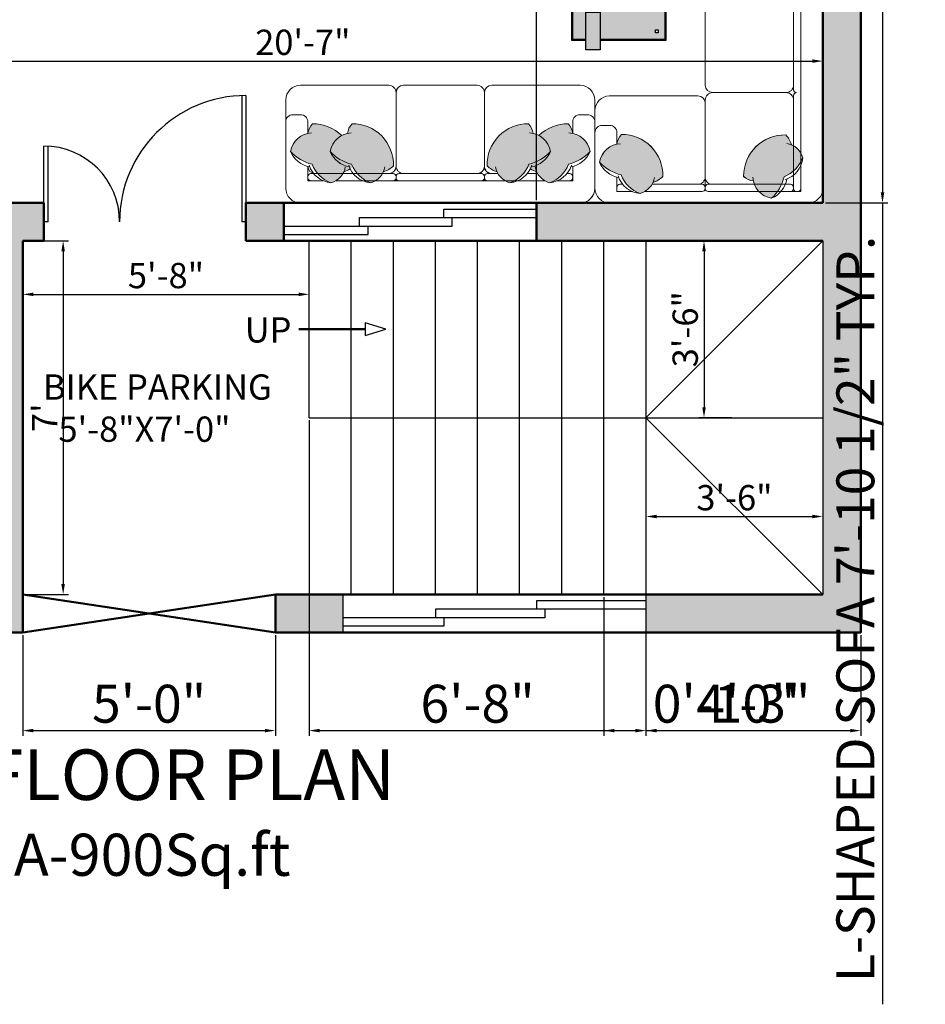
# Model space of a CAD drawing. Units: inches. Extents: x 3274 to 5176, y 1085 to 2172.
# Tile 12 of 16: x 4517 to 4733, y 1085 to 1319. Entities that reach past the tile are written whole.
import ezdxf

# ---------------------------------------------------------------- set-up
doc = ezdxf.new("R2010")
doc.units = ezdxf.units.IN
for name, color, linetype, lineweight in [('A-ANNO-DIMS', 2, 'Continuous', 18), ('A-ANNO-TEXT', 7, 'Continuous', 25), ('A-AREA-IDEN', 3, 'Continuous', 25), ('A-DOOR', 4, 'Continuous', 25), ('A-FLOR-FIXT', 8, 'Continuous', 18), ('A-FLOR-STRS', 7, 'Continuous', 25), ('A-FURN', 8, 'Continuous', 18), ('A-GLAZ', 5, 'Continuous', 25), ('A-WALL', 7, 'Continuous', 50), ('A-WALL-PATT', 8, 'Continuous', 13)]:
    doc.layers.add(name, color=color, linetype=linetype, lineweight=lineweight)
doc.layers.add('MOBIL', color=7, linetype='Continuous')
doc.styles.get("Standard").update_dxf_attribs({"font": 'arial.ttf'})
doc.dimstyles.new('ISO-25', dxfattribs={"dimtxt": 9, "dimasz": 2.5, "dimexe": 1.25, "dimexo": 0.625, "dimtad": 1, "dimdec": 1, "dimlunit": 3, "dimtxsty": 'Standard', "dimcen": 2.5, "dimclrd": 4, "dimclre": 4, "dimclrt": 1, "dimadec": 0, "dimazin": 0, "dimtfac": 1, "dimtdec": 1, "dimtmove": 0, "dimatfit": 3, "dimfxl": 1, "dimarcsym": 0})

# ---------------------------------------------------------------- blocks, each defined once
blk = doc.blocks.new('3')
for p, q in [((47, 30), (47, 0)), ((48, 30), (48, 0)), ((0, 0), (0, 18)), ((1, 0), (1, 18)), ((1, 0), (0, 0)), ((48, 0), (47, 0))]:
    blk.add_line(p, q)
for centre, radius, start, end in [((48, 0), 30, 90, 180), ((0, 0), 18, 0, 90)]:
    blk.add_arc(centre, radius, start, end)
blk = doc.blocks.new('SOFA 1')
at = {"transparency": 33554687}
h = blk.add_hatch(color=256, dxfattribs=at)
h.dxf.hatch_style = 1
h.paths.add_polyline_path([(3769.65, 1307.6, 0.084911), (3767.15, 1309.12, 0.046133), (3766.46, 1311.13), (3759.18, 1311.13, 0.039409), (3758.92, 1310.24, 0.165523), (3756.31, 1309.02, 0.42585), (3767.59, 1297.95, 0.121928), (3769.15, 1300.58, 0.027403), (3769.65, 1300.83)])
h.paths.add_polyline_path([(3765.34, 1313.08), (3760.4, 1313.08, 0.097704), (3759.18, 1311.13), (3766.46, 1311.13, 0.04873)])
h.paths.add_polyline_path([(3763.76, 1314.88, 0.16488), (3760.4, 1313.08), (3765.34, 1313.08, 0.051917)])
h.paths.add_polyline_path([(3771.6, 1305.17, 0.090388), (3769.65, 1307.6), (3769.65, 1300.83, 0.136035), (3771.6, 1302.77)])
h = blk.add_hatch(color=256, dxfattribs=at)
h.dxf.hatch_style = 1
h.paths.add_polyline_path([(3723.52, 1308.63, 0.147724), (3717.76, 1305.24, 0.310469), (3722.42, 1300.4), (3722.42, 1300.25, 0.156703), (3723.62, 1297.8, 0.425821), (3734.69, 1309.08, 0.121928), (3732.05, 1310.63, 0.233216), (3728.6, 1313.59, 0.213835)])
h = blk.add_hatch(color=256, dxfattribs=at)
h.dxf.hatch_style = 1
h.paths.add_polyline_path([(3769.16, 1235.96, 0.122267), (3767.6, 1238.61, 0.425972), (3756.32, 1227.54, 0.165563), (3758.93, 1226.32, 0.309481), (3763.76, 1221.69, 0.002677), (3763.83, 1221.72, 0.146094), (3767.16, 1227.43, 0.212433), (3772.1, 1232.48, 0.235342)])
h = blk.add_hatch(color=256, dxfattribs=at)
h.dxf.hatch_style = 1
h.paths.add_polyline_path([(3769.16, 1225.36, 0.122267), (3767.6, 1228.01, 0.425972), (3756.32, 1216.94, 0.165563), (3758.93, 1215.72, 0.309481), (3763.76, 1211.09, 0.002677), (3763.83, 1211.12, 0.146094), (3767.16, 1216.83, 0.212433), (3772.1, 1221.88, 0.235342)])
for p, q in [((3720.45, 1316.13), (3773.58, 1316.13)), ((3777.51, 1312.19), (3777.51, 1213.72))]:
    blk.add_line(p, q, dxfattribs=at)
for points in [[(3763.76, 1314.88, -0.147724), (3767.15, 1309.12, -0.213355), (3772.1, 1304.05, 0.213355), (3767.15, 1309.12, 0.147724), (3763.76, 1314.88, -0.249545), (3767.86, 1309.77, 0.249545), (3763.77, 1314.89, 0.356779), (3758.8, 1309.23, -0.356779), (3763.76, 1314.88)], [(3717.76, 1305.24, -0.147724), (3723.52, 1308.63, -0.213355), (3728.59, 1313.59, 0.213355), (3723.52, 1308.63, 0.147724), (3717.76, 1305.24, -0.249545), (3722.86, 1309.34, 0.249545), (3717.75, 1305.25, 0.356779), (3723.4, 1300.28, -0.356779), (3717.76, 1305.24)], [(3728.58, 1313.6, -0.306333), (3732.42, 1309.31, 0.306333), (3728.58, 1313.6, 0.306674), (3722.72, 1308.89, -0.306674), (3728.58, 1313.6)], [(3734.69, 1309.08, -0.425972), (3723.62, 1297.8, -0.165552), (3722.4, 1300.4, 0.165552), (3723.62, 1297.79, 0.425972), (3734.69, 1309.07, 0.121514), (3732.07, 1310.63, -0.121514), (3734.69, 1309.08)], [(3767.6, 1297.95, -0.425972), (3756.31, 1309.01, -0.165552), (3758.92, 1310.24, 0.165552), (3756.31, 1309.02, 0.425972), (3767.59, 1297.95, 0.121514), (3769.14, 1300.57, -0.121514), (3767.6, 1297.95)], [(3772.11, 1304.06, -0.306333), (3767.83, 1300.22, 0.306333), (3772.11, 1304.06, 0.306674), (3767.4, 1309.91, -0.306674), (3772.11, 1304.06)], [(3770.44, 1286.63, -0.414214), (3769.66, 1287.4, 0.414214), (3770.44, 1286.63, 0.414214), (3769.66, 1285.83, -0.414214), (3770.44, 1286.63)], [(3748.01, 1262.99, -0.414214), (3746.05, 1264.95, 0.414214), (3748.01, 1262.97, 0.414213), (3746.05, 1261.01, -0.414213), (3748.01, 1262.99)], [(3770.44, 1262.99, -0.414214), (3769.66, 1263.77, 0.414214), (3770.44, 1262.99, 0.414214), (3769.66, 1262.19, -0.414214), (3770.44, 1262.99)], [(3770.83, 1262.97, -0.414214), (3771.61, 1262.19, 0.414214), (3770.83, 1262.99, 0.414214), (3771.61, 1263.77, -0.414214), (3770.83, 1262.97)], [(3748.01, 1239.35, -0.414214), (3746.05, 1241.31, 0.414214), (3748.01, 1239.33, 0.414213), (3746.05, 1237.37, -0.414213), (3748.01, 1239.35)], [(3767.7, 1239.33, -0.414214), (3769.66, 1237.37, 0.414214), (3767.7, 1239.35, 0.414214), (3769.66, 1241.31, -0.414214), (3767.7, 1239.33)], [(3756.32, 1227.54, -0.425972), (3767.6, 1238.61, -0.121514), (3769.16, 1235.98, 0.121514), (3767.6, 1238.61, 0.425972), (3756.32, 1227.54, 0.165552), (3758.93, 1226.32, -0.165552), (3756.32, 1227.54)], [(3770.44, 1239.35, -0.414214), (3769.66, 1240.13, 0.414214), (3770.44, 1239.33, 0.414214), (3769.66, 1238.55, -0.414214), (3770.44, 1239.35)], [(3770.83, 1239.33, -0.414214), (3771.61, 1238.55, 0.414214), (3770.83, 1239.35, 0.414214), (3771.61, 1240.13, -0.414214), (3770.83, 1239.33)], [(3772.1, 1232.5, -0.306674), (3767.41, 1226.64, 0.306674), (3772.1, 1232.5, 0.306333), (3767.84, 1236.34, -0.306333), (3772.1, 1232.5)], [(3763.78, 1221.67, 0.249545), (3767.87, 1226.78, -0.249545), (3763.76, 1221.69, -0.356779), (3758.81, 1227.32, 0.356779), (3763.77, 1221.68, 0.147724), (3767.16, 1227.43, 0.213355), (3772.11, 1232.51, -0.213355), (3767.16, 1227.43, -0.147724), (3763.78, 1221.67)], [(3756.32, 1216.94, -0.200233), (3759.49, 1224.76, 0.200233), (3756.32, 1216.94, 0.165552), (3758.93, 1215.72, -0.165552), (3756.32, 1216.94)], [(3772.1, 1221.9, -0.306674), (3767.41, 1216.04, 0.306674), (3772.1, 1221.9, -0.213355), (3767.16, 1216.83, -0.147724), (3763.77, 1211.08, 0.147724), (3767.15, 1216.83, 0.213355), (3772.1, 1221.9)], [(3763.76, 1211.09, -0.356779), (3758.81, 1216.72, 0.356779), (3763.76, 1211.09, 0.249545), (3767.87, 1216.18, -0.249545), (3763.76, 1211.09)]]:
    blk.add_lwpolyline(points, format="xyb", dxfattribs=at)
for points in [[(3716.51, 1312.2), (3716.51, 1291.44)], [(3722.42, 1313.08), (3722.42, 1309.23), (3722.42, 1313.08), (3726.57, 1313.08)], [(3729.85, 1313.08), (3745.25, 1313.08)], [(3746.01, 1312.3), (3746.01, 1288.55)], [(3768.11, 1313.08), (3746.78, 1313.08)], [(3771.6, 1313.08), (3767.75, 1313.08), (3771.6, 1313.08), (3771.6, 1308.93)], [(3769.66, 1287.39), (3769.65, 1312.3)], [(3771.6, 1313.08), (3771.61, 1233.74)], [(3723.21, 1311.13), (3723.93, 1311.13)], [(3731.82, 1311.13), (3745.25, 1311.13)], [(3746.01, 1310.97), (3746.01, 1311.36)], [(3768.87, 1311.13), (3746.78, 1311.13)], [(3769.65, 1309.43), (3769.65, 1308.71)], [(3746.01, 1288.54), (3746.01, 1308.23)], [(3722.42, 1300.39), (3722.42, 1297.33)], [(3720.45, 1295.38), (3718.48, 1295.38)], [(3720.45, 1287.5), (3744.09, 1287.5)], [(3747.99, 1286.6), (3767.69, 1286.6)], [(3769.66, 1263.75), (3769.66, 1285.81)], [(3746.02, 1284.63), (3746.02, 1264.94)], [(3769.66, 1277.18), (3769.66, 1263.75)], [(3747.99, 1262.97), (3767.69, 1262.97)], [(3769.66, 1240.12), (3769.66, 1262.18)], [(3770.43, 1262.97), (3770.82, 1262.97)], [(3746.02, 1260.99), (3746.02, 1241.3)], [(3747.99, 1239.33), (3767.69, 1239.33)], [(3769.66, 1235.71), (3769.66, 1238.54)], [(3770.43, 1239.33), (3770.82, 1239.33)], [(3746.02, 1237.36), (3746.02, 1213.74)], [(3771.61, 1223.14), (3771.61, 1230.47)], [(3769.66, 1225.11), (3769.66, 1227.82)], [(3767.76, 1215.72), (3771.61, 1215.72), (3771.61, 1219.84), (3771.61, 1215.72)], [(3769.66, 1216.5), (3769.66, 1217.22)], [(3755.86, 1215.72), (3758.92, 1215.72)], [(3753.91, 1211.77), (3753.91, 1213.74)], [(3749.97, 1209.8), (3773.58, 1209.8)]]:
    blk.add_lwpolyline(points, close=True, dxfattribs=at)
for points in [[(3722.42, 1311.91, 0.414214), (3723.2, 1311.13, -0.414214)], [(3770.43, 1313.08, 0.414214), (3769.65, 1312.3, -0.414214)], [(3771.6, 1312.3, 0.414214), (3770.82, 1313.08, -0.414214)], [(3716.51, 1297.34, 0.414214), (3718.47, 1295.38, -0.414214)], [(3720.44, 1295.38, 0.414214), (3722.4, 1297.34, -0.414214)], [(3716.51, 1291.45, 0.414212), (3720.44, 1287.52, -0.414212)], [(3746.03, 1288.56, 0.414214), (3747.99, 1286.6, 0.414213), (3746.03, 1284.64, -0.414213), (3747.99, 1286.6, -0.414214)], [(3769.66, 1284.64, 0.414214), (3767.7, 1286.6, 0.414214), (3769.66, 1288.56, -0.414214), (3767.7, 1286.6, -0.414214)], [(3769.66, 1261.01, 0.414214), (3767.7, 1262.97, 0.414214), (3769.66, 1264.93, -0.414214), (3767.7, 1262.97, -0.414214)], [(3772.13, 1221.9, 0.306333), (3767.84, 1225.74, -0.306333)], [(3769.16, 1225.36, 0.071861), (3768.39, 1227.01, -0.071861)], [(3755.87, 1215.72, 0.414214), (3753.91, 1213.76, -0.414214)], [(3769.66, 1216.52, 0.414214), (3770.44, 1215.74, -0.414214)], [(3770.83, 1215.74, 0.414214), (3771.61, 1216.52, -0.414214)], [(3746.05, 1213.76, 0.414212), (3749.98, 1209.82, -0.414212)], [(3755.87, 1209.8, -0.414214), (3753.91, 1211.76, 0.414214)]]:
    blk.add_lwpolyline(points, format="xyb", close=True, dxfattribs=at)
for centre, radius, start, end in [((3720.44, 1312.2), 3.93, 90.0002, 179.9998), ((3720.44, 1312.19), 3.94, 89.9158, 179.9154), ((3773.58, 1312.2), 3.93, 0.0002, 89.9998), ((3773.57, 1312.19), 3.94, 359.9158, 89.9154), ((3745.22, 1312.29), 0.789, 0.8425, 90.8425), ((3745.24, 1311.91), 0.777, 270, 0), ((3745.24, 1311.91), 0.777, 270, 0), ((3746.8, 1312.29), 0.789, 89.1575, 179.1575), ((3746.79, 1311.91), 0.777, 180, 270), ((3746.79, 1311.91), 0.777, 180, 270), ((3768.87, 1312.3), 0.777, 360, 90), ((3768.87, 1311.91), 0.777, 270, 0), ((3744.09, 1309.21), 1.92, 358.766, 90.5111), ((3747.93, 1309.21), 1.92, 89.4889, 181.234), ((3744.08, 1289.48), 1.96, 270, 360), ((3744.08, 1289.48), 1.96, 270, 360), ((3773.58, 1213.73), 3.93, 270.0002, 359.9998), ((3773.59, 1213.73), 3.93, 269.9156, 359.9152)]:
    blk.add_arc(centre, radius, start, end, dxfattribs=at)
blk = doc.blocks.new('Mesa de centro Cantria feeling')
at = {"layer": 'MOBIL', "ltscale": 0.2}
h = blk.add_hatch(color=256, dxfattribs=at)
h.set_gradient(color1=(74, 55, 38), color2=(104, 77, 54), one_color=1, tint=0.31, name='CYLINDER')
h.paths.add_polyline_path([(-0.85, -0.3), (-0.7, -0.3), (-0.7, 0.1), (-0.85, 0.1)])
h = blk.add_hatch(color=256, dxfattribs=at)
h.set_gradient(color1=(221, 221, 223), one_color=1, tint=1)
h.paths.add_polyline_path([(-0.15, -0.6), (-0.15, -0.89), (-0.01, -0.89), (-0.01, -0.01), (-0.7, -0.01), (-0.7, -0.3), (-0.85, -0.3), (-0.85, -0.01), (-0.99, -0.01), (-0.99, -0.89), (-0.3, -0.89), (-0.3, -0.6)])
h.paths.add_polyline_path([(-0.112, -0.112), (-0.112, -0.082), (-0.082, -0.082), (-0.082, -0.112)], flags=16)
h.paths.add_polyline_path([(-0.888, -0.788), (-0.888, -0.818), (-0.918, -0.818), (-0.918, -0.788)], flags=16)
h = blk.add_hatch(color=256, dxfattribs=at)
h.set_gradient(color1=(74, 55, 38), color2=(104, 77, 54), one_color=1, tint=0.31, name='CYLINDER')
h.paths.add_polyline_path([(-0.15, -0.6), (-0.3, -0.6), (-0.3, -1), (-0.15, -1)])
for points in [[(-0.85, 0), (-1, 0), (-1, -0.9), (-0.3, -0.9)], [(-0.15, -0.9), (0, -0.9), (0, 0), (-0.7, 0)], [(-0.85, -0.01), (-0.99, -0.01), (-0.99, -0.89), (-0.3, -0.89)], [(-0.15, -0.89), (-0.01, -0.89), (-0.01, -0.01), (-0.7, -0.01)]]:
    blk.add_lwpolyline(points, dxfattribs=at)
for points in [[(-0.85, -0.3), (-0.7, -0.3), (-0.7, 0.1), (-0.85, 0.1)], [(-0.082, -0.082), (-0.112, -0.082), (-0.112, -0.112), (-0.082, -0.112)], [(-0.15, -0.6), (-0.3, -0.6), (-0.3, -1), (-0.15, -1)], [(-0.918, -0.818), (-0.888, -0.818), (-0.888, -0.788), (-0.918, -0.788)]]:
    blk.add_lwpolyline(points, close=True, dxfattribs=at)
blk = doc.blocks.new('S1')
at = {"transparency": 33554687}
h = blk.add_hatch(color=256, dxfattribs=at)
h.dxf.hatch_style = 1
h.paths.add_polyline_path([(3706.22, 1117.89, 0.122267), (3708.57, 1119.27, 0.425972), (3698.75, 1129.29, 0.165563), (3697.66, 1126.97, 0.309481), (3693.55, 1122.68, 0.002677), (3693.58, 1122.62, 0.146094), (3698.65, 1119.67, 0.212433), (3703.13, 1115.28, 0.235342)])
h = blk.add_hatch(color=256, dxfattribs=at)
h.dxf.hatch_style = 1
h.paths.add_polyline_path([(3715.63, 1117.89, 0.122267), (3717.98, 1119.27, 0.425972), (3708.16, 1129.29, 0.165563), (3707.07, 1126.97, 0.309481), (3702.96, 1122.68, 0.002677), (3702.99, 1122.62, 0.146094), (3708.06, 1119.67, 0.212433), (3712.54, 1115.28, 0.235342)])
h = blk.add_hatch(color=256, dxfattribs=at)
h.dxf.hatch_style = 1
h.paths.add_polyline_path([(3742.59, 1117.89, -0.122267), (3740.24, 1119.27, -0.425972), (3750.07, 1129.29, -0.165563), (3751.15, 1126.97, -0.309481), (3755.26, 1122.68, -0.002677), (3755.24, 1122.62, -0.146094), (3750.16, 1119.67, -0.212433), (3745.68, 1115.28, -0.235342)])
h = blk.add_hatch(color=256, dxfattribs=at)
h.dxf.hatch_style = 1
h.paths.add_polyline_path([(3752, 1117.89, -0.122267), (3749.65, 1119.27, -0.425972), (3759.48, 1129.29, -0.165563), (3760.56, 1126.97, -0.309481), (3764.67, 1122.68, -0.002677), (3764.65, 1122.62, -0.146094), (3759.57, 1119.67, -0.212433), (3755.09, 1115.28, -0.235342)])
for p, q in [((3747.47, 1115.72), (3704.36, 1115.76)), ((3695.9, 1110.48), (3762.33, 1110.48))]:
    blk.add_line(p, q)
for points in [[(3695.92, 1138.41, 0.414212), (3692.43, 1134.92, -0.414212)], [(3762.3, 1138.41, -0.414212), (3765.79, 1134.92, 0.414212)], [(3692.41, 1129.69, -0.414214), (3694.15, 1131.43, 0.414214)], [(3697.66, 1129.69, 0.414214), (3695.92, 1131.43, -0.414214)], [(3760.56, 1129.69, -0.414214), (3762.3, 1131.43, 0.414214)], [(3765.81, 1129.69, 0.414214), (3764.07, 1131.43, -0.414214)], [(3703.15, 1115.26, 0.306333), (3706.55, 1119.07, -0.306333)], [(3706.22, 1117.89, 0.071861), (3707.68, 1118.58, -0.071861)], [(3720.36, 1117.45, -0.414214), (3718.62, 1119.19, -0.414214), (3716.88, 1117.45, 0.414214), (3718.62, 1119.19, 0.414214)], [(3752, 1117.89, -0.071861), (3750.54, 1118.58, 0.071861)], [(3755.08, 1115.26, -0.306333), (3751.67, 1119.07, 0.306333)], [(3698.37, 1117.45, 0.414214), (3697.68, 1116.76, -0.414214)], [(3697.68, 1116.41, 0.414214), (3698.37, 1115.72, -0.414214)], [(3759.85, 1117.45, -0.414214), (3760.54, 1116.76, 0.414214)], [(3760.54, 1116.41, -0.414214), (3759.85, 1115.72, 0.414214)]]:
    blk.add_lwpolyline(points, format="xyb", close=True, dxfattribs=at)
for points in [[(3695.92, 1138.41), (3716.87, 1138.43)], [(3718.62, 1136.68), (3718.62, 1119.2)], [(3720.37, 1138.43), (3737.85, 1138.43)], [(3739.6, 1136.68), (3739.6, 1119.2)], [(3741.35, 1138.43), (3762.31, 1138.43)], [(3692.41, 1134.93), (3692.41, 1113.97)], [(3692.41, 1134.81), (3692.41, 1113.85)], [(3765.81, 1134.93), (3765.81, 1113.97)], [(3694.16, 1131.43), (3695.91, 1131.43)], [(3697.66, 1129.7), (3697.66, 1126.98)], [(3760.56, 1129.7), (3760.56, 1126.98)], [(3764.06, 1131.43), (3762.31, 1131.43)], [(3697.66, 1119.14), (3697.66, 1115.72), (3701.32, 1115.72), (3697.66, 1115.72)], [(3760.56, 1119.14), (3760.56, 1115.72), (3756.9, 1115.72), (3760.56, 1115.72)], [(3717.92, 1117.45), (3698.34, 1117.45)], [(3698.35, 1117.46), (3698.99, 1117.46)], [(3698.36, 1117.45), (3699, 1117.45)], [(3706, 1117.45), (3717.92, 1117.45)], [(3718.62, 1116.77), (3718.62, 1116.42)], [(3738.9, 1117.45), (3719.32, 1117.45)], [(3739.6, 1116.77), (3739.6, 1116.42)], [(3742.81, 1117.45), (3740.3, 1117.45)], [(3753.97, 1115.72), (3747.47, 1115.72)], [(3752.22, 1117.45), (3749.81, 1117.45)], [(3759.86, 1117.45), (3759.22, 1117.45)]]:
    blk.add_lwpolyline(points, close=True, dxfattribs=at)
for points in [[(3718.6, 1136.67, 0.414214), (3716.86, 1138.41, -0.414214), (3718.62, 1136.67, -0.414213), (3720.36, 1138.41, 0.414213), (3718.6, 1136.67)], [(3739.58, 1136.67, 0.414214), (3737.84, 1138.41, -0.414214), (3739.6, 1136.67, -0.414213), (3741.34, 1138.41, 0.414213), (3739.58, 1136.67)], [(3698.75, 1129.29, -0.200233), (3705.69, 1126.47, 0.200233), (3698.75, 1129.29, 0.165552), (3697.66, 1126.97, -0.165552), (3698.75, 1129.29)], [(3708.16, 1129.29, -0.425972), (3717.98, 1119.27, -0.121514), (3715.65, 1117.89, 0.121514), (3717.98, 1119.27, 0.425972), (3708.16, 1129.29, 0.165552), (3707.07, 1126.97, -0.165552), (3708.16, 1129.29)], [(3750.07, 1129.29, 0.425972), (3740.24, 1119.27, 0.121514), (3742.57, 1117.89, -0.121514), (3740.24, 1119.27, -0.425972), (3750.07, 1129.29, -0.165552), (3751.15, 1126.97, 0.165552), (3750.07, 1129.29)], [(3759.48, 1129.29, 0.200233), (3752.53, 1126.47, -0.200233), (3759.48, 1129.29, -0.165552), (3760.56, 1126.97, 0.165552), (3759.48, 1129.29)], [(3693.55, 1122.68, -0.356779), (3698.55, 1127.08, 0.356779), (3693.55, 1122.68, 0.249545), (3698.07, 1119.04, -0.249545), (3693.55, 1122.68)], [(3702.94, 1122.67, 0.249545), (3707.48, 1119.04, -0.249545), (3702.96, 1122.68, -0.356779), (3707.96, 1127.08, 0.356779), (3702.95, 1122.67, 0.147724), (3708.06, 1119.67, 0.213355), (3712.56, 1115.27, -0.213355), (3708.06, 1119.67, -0.147724), (3702.94, 1122.67)], [(3755.28, 1122.67, -0.249545), (3750.74, 1119.04, 0.249545), (3755.26, 1122.68, 0.356779), (3750.26, 1127.08, -0.356779), (3755.27, 1122.67, -0.147724), (3750.16, 1119.67, -0.213355), (3745.66, 1115.27, 0.213355), (3750.16, 1119.67, 0.147724), (3755.28, 1122.67)], [(3764.67, 1122.68, 0.356779), (3759.67, 1127.08, -0.356779), (3764.67, 1122.68, -0.249545), (3760.15, 1119.04, 0.249545), (3764.67, 1122.68)], [(3703.15, 1115.28, -0.306674), (3697.95, 1119.44, 0.306674), (3703.15, 1115.28, -0.213355), (3698.65, 1119.67, -0.147724), (3693.54, 1122.67, 0.147724), (3698.65, 1119.67, 0.213355), (3703.15, 1115.28)], [(3755.07, 1115.28, 0.306674), (3760.27, 1119.44, -0.306674), (3755.07, 1115.28, 0.213355), (3759.57, 1119.67, 0.147724), (3764.68, 1122.67, -0.147724), (3759.57, 1119.67, -0.213355), (3755.07, 1115.28)], [(3712.56, 1115.28, -0.306674), (3707.36, 1119.44, 0.306674), (3712.56, 1115.28, 0.306333), (3715.96, 1119.07, -0.306333), (3712.56, 1115.28)], [(3739.6, 1119.19, 0.414214), (3741.34, 1117.45, -0.414214), (3739.58, 1119.19, -0.414214), (3737.84, 1117.45, 0.414214), (3739.6, 1119.19)], [(3745.66, 1115.28, 0.306674), (3750.86, 1119.44, -0.306674), (3745.66, 1115.28, -0.306333), (3742.26, 1119.07, 0.306333), (3745.66, 1115.28)], [(3718.6, 1116.76, 0.414214), (3717.91, 1117.45, -0.414214), (3718.6, 1116.76, -0.414214), (3719.31, 1117.45, 0.414214), (3718.6, 1116.76)], [(3718.62, 1116.41, 0.414214), (3719.31, 1115.72, -0.414214), (3718.6, 1116.41, -0.414214), (3717.91, 1115.72, 0.414214), (3718.62, 1116.41)], [(3739.58, 1116.76, 0.414214), (3738.89, 1117.45, -0.414214), (3739.6, 1116.76, -0.414214), (3740.29, 1117.45, 0.414214), (3739.58, 1116.76)], [(3739.6, 1116.41, 0.414214), (3740.29, 1115.72, -0.414214), (3739.58, 1116.41, -0.414214), (3738.89, 1115.72, 0.414214), (3739.6, 1116.41)]]:
    blk.add_lwpolyline(points, format="xyb", dxfattribs=at)
for centre, radius, start, end in [((3699.38, 1119.19), 1.74, 180, 270), ((3699.38, 1119.19), 1.74, 180, 270), ((3695.9, 1113.97), 3.5, 180.0846, 270.0842), ((3762.32, 1113.97), 3.49, 270.0002, 359.9998), ((3762.33, 1113.96), 3.48, 270.0848, 0.0844)]:
    blk.add_arc(centre, radius, start, end, dxfattribs=at)
blk = doc.blocks.new('*D77')
at = {"layer": 'A-ANNO-DIMS', "color": 0, "lineweight": -2, "transparency": 16777216}
for p, q in [((4518.81, 1266.35), (4529.02, 1266.35)), ((4527.77, 1263.85), (4527.77, 1184.85)), ((4518.81, 1182.35), (4529.02, 1182.35))]:
    blk.add_line(p, q, dxfattribs=at)
at = {"layer": 'A-ANNO-DIMS', "color": 0, "transparency": 16777216}
for points in [[(4527.35, 1263.85), (4528.19, 1263.85), (4527.77, 1266.35)], [(4527.35, 1184.85), (4528.19, 1184.85), (4527.77, 1182.35)]]:
    blk.add_solid(points, dxfattribs=at)
at = {"layer": 'Defpoints', "color": 0, "transparency": 16777216}
for p in [(4518.19, 1266.35), (4518.19, 1182.35), (4527.77, 1182.35)]:
    blk.add_point(p, dxfattribs=at)
at = {"layer": 'A-ANNO-DIMS', "color": 0, "transparency": 16777216, "insert": (4524.15, 1224.35), "char_height": 6, "attachment_point": 5, "rotation": 90}
blk.add_mtext("7'", dxfattribs=at)
blk = doc.blocks.new('*D78')
at = {"layer": 'A-ANNO-DIMS', "color": 0, "lineweight": -2, "transparency": 16777216}
for p, q in [((4520.69, 1253.63), (4583.69, 1253.63)), ((4586.19, 1254.26), (4586.19, 1254.88)), ((4518.19, 1253.01), (4518.19, 1252.38))]:
    blk.add_line(p, q, dxfattribs=at)
at = {"layer": 'A-ANNO-DIMS', "color": 0, "transparency": 16777216}
for points in [[(4520.69, 1254.05), (4520.69, 1253.22), (4518.19, 1253.63)], [(4583.69, 1254.05), (4583.69, 1253.22), (4586.19, 1253.63)]]:
    blk.add_solid(points, dxfattribs=at)
at = {"layer": 'Defpoints', "color": 0, "transparency": 16777216}
for p in [(4518.19, 1253.63), (4586.19, 1253.63), (4586.19, 1253.63)]:
    blk.add_point(p, dxfattribs=at)
at = {"layer": 'A-ANNO-DIMS', "color": 0, "transparency": 16777216, "insert": (4552.19, 1257.32), "char_height": 6, "attachment_point": 5}
blk.add_mtext('5\'-8"', dxfattribs=at)
blk = doc.blocks.new('*D79')
at = {"layer": 'A-ANNO-DIMS', "color": 0, "lineweight": -2, "transparency": 16777216}
for p, q in [((4686.6, 1266.35), (4678.72, 1266.35)), ((4679.97, 1263.85), (4679.97, 1226.85)), ((4686.6, 1224.35), (4678.72, 1224.35))]:
    blk.add_line(p, q, dxfattribs=at)
at = {"layer": 'A-ANNO-DIMS', "color": 0, "transparency": 16777216}
for points in [[(4679.56, 1263.85), (4680.39, 1263.85), (4679.97, 1266.35)], [(4679.56, 1226.85), (4680.39, 1226.85), (4679.97, 1224.35)]]:
    blk.add_solid(points, dxfattribs=at)
at = {"layer": 'Defpoints', "color": 0, "transparency": 16777216}
for p in [(4687.22, 1266.35), (4679.97, 1224.35), (4687.22, 1224.35)]:
    blk.add_point(p, dxfattribs=at)
at = {"layer": 'A-ANNO-DIMS', "color": 0, "transparency": 16777216, "insert": (4676.28, 1245.35), "char_height": 6, "attachment_point": 5, "rotation": 90}
blk.add_mtext('3\'-6"', dxfattribs=at)
blk = doc.blocks.new('*D80')
at = {"layer": 'A-ANNO-DIMS', "color": 0, "lineweight": -2, "transparency": 16777216}
for p, q in [((4666.19, 1204.4), (4666.19, 1199.64)), ((4708.19, 1204.4), (4708.19, 1199.64)), ((4668.69, 1200.89), (4705.69, 1200.89))]:
    blk.add_line(p, q, dxfattribs=at)
at = {"layer": 'A-ANNO-DIMS', "color": 0, "transparency": 16777216}
for points in [[(4668.69, 1201.31), (4668.69, 1200.47), (4666.19, 1200.89)], [(4705.69, 1201.31), (4705.69, 1200.47), (4708.19, 1200.89)]]:
    blk.add_solid(points, dxfattribs=at)
at = {"layer": 'Defpoints', "color": 0, "transparency": 16777216}
for p in [(4666.19, 1205.03), (4708.19, 1205.03), (4708.19, 1200.89)]:
    blk.add_point(p, dxfattribs=at)
at = {"layer": 'A-ANNO-DIMS', "color": 0, "transparency": 16777216, "insert": (4687.19, 1204.58), "char_height": 6, "attachment_point": 5}
blk.add_mtext('3\'-6"', dxfattribs=at)
blk = doc.blocks.new('*D81')
at = {"layer": 'A-ANNO-DIMS', "color": 0, "lineweight": -2, "transparency": 16777216}
for p, q in [((4461.19, 1312.95), (4461.19, 1307.77)), ((4708.19, 1312.95), (4708.19, 1307.77)), ((4463.69, 1309.02), (4705.69, 1309.02))]:
    blk.add_line(p, q, dxfattribs=at)
at = {"layer": 'A-ANNO-DIMS', "color": 0, "transparency": 16777216}
for points in [[(4463.69, 1309.44), (4463.69, 1308.61), (4461.19, 1309.02)], [(4705.69, 1309.44), (4705.69, 1308.61), (4708.19, 1309.02)]]:
    blk.add_solid(points, dxfattribs=at)
at = {"layer": 'Defpoints', "color": 0, "transparency": 16777216}
for p in [(4461.19, 1313.57), (4708.19, 1313.57), (4708.19, 1309.02)]:
    blk.add_point(p, dxfattribs=at)
at = {"layer": 'A-ANNO-DIMS', "color": 0, "transparency": 16777216, "insert": (4584.69, 1312.71), "char_height": 6, "attachment_point": 5}
blk.add_mtext('20\'-7"', dxfattribs=at)
blk = doc.blocks.new('WIN-60')
for p, q in [((4598.19, 1271.85), (4640.19, 1271.85)), ((4598.19, 1269.85), (4598.19, 1271.85)), ((4618.19, 1273.85), (4640.19, 1273.85)), ((4618.19, 1271.85), (4618.19, 1273.85)), ((4620.19, 1269.85), (4620.19, 1271.85)), ((4580.19, 1269.85), (4620.19, 1269.85)), ((4600.19, 1267.85), (4600.19, 1269.85)), ((4580.19, 1267.85), (4600.19, 1267.85))]:
    blk.add_line(p, q)
blk = doc.blocks.new('WIN-72')
for p, q in [((4462.19, 1180.85), (4436.19, 1180.85)), ((4436.19, 1180.85), (4436.19, 1178.85)), ((4462.19, 1178.85), (4412.19, 1178.85)), ((4412.19, 1178.85), (4412.19, 1176.85)), ((4438.19, 1178.85), (4438.19, 1176.85)), ((4438.19, 1176.85), (4390.19, 1176.85)), ((4414.19, 1176.85), (4414.19, 1174.85)), ((4414.19, 1174.85), (4390.19, 1174.85))]:
    blk.add_line(p, q)
blk = doc.blocks.new('*D136')
at = {"layer": 'A-ANNO-DIMS', "color": 4, "lineweight": -2, "transparency": 16777216}
for p, q in [((4708.83, 1369.73), (4723.61, 1369.73)), ((4722.36, 1367.23), (4722.36, 1277.84)), ((4708.83, 1275.34), (4723.61, 1275.34)), ((4722.36, 1275.34), (4722.36, 1085.06))]:
    blk.add_line(p, q, dxfattribs=at)
at = {"layer": 'A-ANNO-DIMS', "color": 4, "transparency": 16777216}
for points in [[(4721.94, 1367.23), (4722.78, 1367.23), (4722.36, 1369.73)], [(4721.94, 1277.84), (4722.78, 1277.84), (4722.36, 1275.34)]]:
    blk.add_solid(points, dxfattribs=at)
at = {"layer": 'Defpoints', "color": 0, "transparency": 16777216}
for p in [(4708.2, 1369.73), (4708.2, 1275.34), (4722.36, 1275.34)]:
    blk.add_point(p, dxfattribs=at)
at = {"layer": 'A-ANNO-DIMS', "color": 1, "transparency": 16777216, "insert": (4717.08, 1178.95), "char_height": 9, "attachment_point": 5, "rotation": 90}
blk.add_mtext('L-SHAPED SOFA 7\'-10 1/2" TYP.', dxfattribs=at)
blk = doc.blocks.new('*D148')
at = {"layer": 'A-ANNO-DIMS', "color": 4, "lineweight": -2, "transparency": 16777216}
for p, q in [((4666.19, 1172.73), (4666.19, 1148.8)), ((4717.19, 1172.73), (4717.19, 1148.8)), ((4668.69, 1150.05), (4714.69, 1150.05))]:
    blk.add_line(p, q, dxfattribs=at)
at = {"layer": 'A-ANNO-DIMS', "color": 4, "transparency": 16777216}
for points in [[(4668.69, 1150.47), (4668.69, 1149.64), (4666.19, 1150.05)], [(4714.69, 1150.47), (4714.69, 1149.64), (4717.19, 1150.05)]]:
    blk.add_solid(points, dxfattribs=at)
at = {"layer": 'Defpoints', "color": 0, "transparency": 16777216}
for p in [(4666.19, 1173.35), (4717.19, 1173.35), (4717.19, 1150.05)]:
    blk.add_point(p, dxfattribs=at)
at = {"layer": 'A-ANNO-DIMS', "color": 1, "transparency": 16777216, "insert": (4691.69, 1155.28), "char_height": 9, "attachment_point": 5}
blk.add_mtext('4\'-3"', dxfattribs=at)
blk = doc.blocks.new('*D149')
at = {"layer": 'A-ANNO-DIMS', "color": 4, "lineweight": -2, "transparency": 16777216}
for p, q in [((4518.19, 1172.73), (4518.19, 1148.8)), ((4578.19, 1172.73), (4578.19, 1148.8)), ((4520.69, 1150.05), (4575.69, 1150.05))]:
    blk.add_line(p, q, dxfattribs=at)
at = {"layer": 'A-ANNO-DIMS', "color": 4, "transparency": 16777216}
for points in [[(4520.69, 1150.47), (4520.69, 1149.64), (4518.19, 1150.05)], [(4575.69, 1150.47), (4575.69, 1149.64), (4578.19, 1150.05)]]:
    blk.add_solid(points, dxfattribs=at)
at = {"layer": 'Defpoints', "color": 0, "transparency": 16777216}
for p in [(4518.19, 1173.35), (4578.19, 1173.35), (4578.19, 1150.05)]:
    blk.add_point(p, dxfattribs=at)
at = {"layer": 'A-ANNO-DIMS', "color": 1, "transparency": 16777216, "insert": (4548.19, 1155.27), "char_height": 9, "attachment_point": 5}
blk.add_mtext('5\'-0"', dxfattribs=at)
blk = doc.blocks.new('*D152')
at = {"layer": 'A-ANNO-DIMS', "color": 4, "lineweight": -2, "transparency": 16777216}
for p, q in [((4586.19, 1223.73), (4586.19, 1148.8)), ((4666.19, 1223.73), (4666.19, 1148.8)), ((4588.69, 1150.05), (4663.69, 1150.05))]:
    blk.add_line(p, q, dxfattribs=at)
at = {"layer": 'A-ANNO-DIMS', "color": 4, "transparency": 16777216}
for points in [[(4588.69, 1150.47), (4588.69, 1149.64), (4586.19, 1150.05)], [(4663.69, 1150.47), (4663.69, 1149.64), (4666.19, 1150.05)]]:
    blk.add_solid(points, dxfattribs=at)
at = {"layer": 'Defpoints', "color": 0, "transparency": 16777216}
for p in [(4586.19, 1224.35), (4666.19, 1224.35), (4666.19, 1150.05)]:
    blk.add_point(p, dxfattribs=at)
at = {"layer": 'A-ANNO-DIMS', "color": 1, "transparency": 16777216, "insert": (4626.19, 1155.27), "char_height": 9, "attachment_point": 5}
blk.add_mtext('6\'-8"', dxfattribs=at)
blk = doc.blocks.new('*D153')
at = {"layer": 'A-ANNO-DIMS', "color": 4, "lineweight": -2, "transparency": 16777216}
for p, q in [((4656.19, 1181.73), (4656.19, 1148.8)), ((4666.19, 1181.73), (4666.19, 1148.8)), ((4658.69, 1150.05), (4663.69, 1150.05)), ((4666.19, 1150.05), (4700.85, 1150.05))]:
    blk.add_line(p, q, dxfattribs=at)
at = {"layer": 'A-ANNO-DIMS', "color": 4, "transparency": 16777216}
for points in [[(4658.69, 1150.47), (4658.69, 1149.64), (4656.19, 1150.05)], [(4663.69, 1150.47), (4663.69, 1149.64), (4666.19, 1150.05)]]:
    blk.add_solid(points, dxfattribs=at)
at = {"layer": 'Defpoints', "color": 0, "transparency": 16777216}
for p in [(4656.19, 1182.35), (4666.19, 1182.35), (4666.19, 1150.05)]:
    blk.add_point(p, dxfattribs=at)
at = {"layer": 'A-ANNO-DIMS', "color": 1, "transparency": 16777216, "insert": (4684.77, 1155.27), "char_height": 9, "attachment_point": 5}
blk.add_mtext('0\'-10"', dxfattribs=at)
blk = doc.blocks.new('*D154')
at = {"layer": 'A-ANNO-DIMS', "color": 4, "lineweight": -2, "transparency": 16777216}
for p, q in [((4640.19, 1275.98), (4640.19, 1557.9)), ((4708.19, 1275.98), (4708.19, 1557.9)), ((4642.69, 1556.65), (4705.69, 1556.65))]:
    blk.add_line(p, q, dxfattribs=at)
at = {"layer": 'A-ANNO-DIMS', "color": 4, "transparency": 16777216}
for points in [[(4642.69, 1557.07), (4642.69, 1556.24), (4640.19, 1556.65)], [(4705.69, 1557.07), (4705.69, 1556.24), (4708.19, 1556.65)]]:
    blk.add_solid(points, dxfattribs=at)
at = {"layer": 'Defpoints', "color": 0, "transparency": 16777216}
for p in [(4708.19, 1556.65), (4640.19, 1275.35), (4708.19, 1275.35)]:
    blk.add_point(p, dxfattribs=at)
at = {"layer": 'A-ANNO-DIMS', "color": 1, "transparency": 16777216, "insert": (4674.19, 1561.87), "char_height": 9, "attachment_point": 5}
blk.add_mtext('5\'-8"', dxfattribs=at)

msp = doc.modelspace()

# ---------------------------------------------------------------- hatches: boundary and pattern name
at = {"layer": 'A-WALL-PATT'}
h = msp.add_hatch(color=256, dxfattribs=at)
h.dxf.hatch_style = 1
h.paths.add_polyline_path([(4717.19, 1533.35), (4357.19, 1533.35), (4357.19, 1173.35), (4390.19, 1173.35), (4390.19, 1182.35), (4366.19, 1182.35), (4366.19, 1266.35), (4426.19, 1266.35), (4426.19, 1271.35), (4366.19, 1271.35), (4366.19, 1375.35), (4426.19, 1375.35), (4426.19, 1380.35), (4366.19, 1380.35), (4366.19, 1524.35), (4708.19, 1524.35), (4708.19, 1380.35), (4578.19, 1380.35), (4578.19, 1375.35), (4708.19, 1375.35), (4708.19, 1275.35), (4640.19, 1275.35), (4640.19, 1266.35), (4708.19, 1266.35), (4708.19, 1182.35), (4666.19, 1182.35), (4666.19, 1173.35), (4717.19, 1173.35)])
h.paths.add_polyline_path([(4461.19, 1375.35), (4477.19, 1375.35), (4477.19, 1380.35), (4456.19, 1380.35), (4456.19, 1319.35), (4401.19, 1319.35), (4401.19, 1339.35), (4396.19, 1339.35), (4396.19, 1314.35), (4456.19, 1314.35), (4456.19, 1266.35), (4477.19, 1266.35), (4477.19, 1271.35), (4461.19, 1271.35)], flags=17)
h.paths.add_polyline_path([(4518.19, 1483.35), (4536.19, 1483.35), (4536.19, 1488.35), (4513.19, 1488.35), (4513.19, 1375.35), (4536.19, 1375.35), (4536.19, 1380.35), (4518.19, 1380.35), (4518.19, 1418.35), (4548.19, 1418.35), (4548.19, 1423.35), (4518.19, 1423.35)], flags=17)
h.paths.add_polyline_path([(4583.19, 1488.35), (4560.19, 1488.35), (4560.19, 1483.35), (4578.19, 1483.35), (4578.19, 1416.35), (4583.19, 1416.35)], flags=17)
h.paths.add_polyline_path([(4518.19, 1266.35), (4523.19, 1266.35), (4523.19, 1275.35), (4513.19, 1275.35), (4513.19, 1182.35), (4462.19, 1182.35), (4462.19, 1173.35), (4518.19, 1173.35)], flags=17)
h.paths.add_polyline_path([(4580.19, 1275.35), (4571.19, 1275.35), (4571.19, 1270.85), (4571.19, 1266.35), (4580.19, 1266.35)], flags=17)
h.paths.add_polyline_path([(4594.19, 1182.35), (4578.19, 1182.35), (4578.19, 1173.35), (4594.19, 1173.35)], flags=17)
h.paths.add_polyline_path([(4573.24, 1316.29), (4647.44, 1316.29), (4647.44, 1346.14), (4573.24, 1346.14)], flags=25)
h.paths.add_polyline_path([(4529.43, 1453), (4568.61, 1453), (4568.61, 1475.39), (4529.43, 1475.39)], flags=25)
h.paths.add_polyline_path([(4619, 1443.76), (4687.39, 1443.76), (4687.39, 1473.61), (4619, 1473.61)], flags=25)
h.paths.add_polyline_path([(4527.67, 1497.04), (4569.64, 1497.04), (4569.64, 1519.43), (4527.67, 1519.43)], flags=25)
h.paths.add_polyline_path([(4407.08, 1443.76), (4475.47, 1443.76), (4475.47, 1473.61), (4407.08, 1473.61)], flags=25)

# ---------------------------------------------------------------- linework, layer by layer
at = {"layer": 'A-FLOR-STRS'}
for p, q in [((4586.19, 1224.35), (4586.19, 1266.35)), ((4596.19, 1224.35), (4596.19, 1266.35)), ((4606.19, 1224.35), (4606.19, 1266.35)), ((4616.19, 1224.35), (4616.19, 1266.35)), ((4626.19, 1224.35), (4626.19, 1266.35)), ((4636.19, 1224.35), (4636.19, 1266.35)), ((4646.19, 1224.35), (4646.19, 1266.35)), ((4656.19, 1224.35), (4656.19, 1266.35)), ((4666.19, 1266.35), (4666.19, 1182.35)), ((4666.19, 1224.35), (4708.19, 1266.35)), ((4708.19, 1266.35), (4708.19, 1182.35)), ((4586.19, 1224.35), (4708.19, 1224.35)), ((4596.19, 1182.35), (4596.19, 1224.35)), ((4606.19, 1182.35), (4606.19, 1224.35)), ((4616.19, 1182.35), (4616.19, 1224.35)), ((4626.19, 1182.35), (4626.19, 1224.35)), ((4636.19, 1182.35), (4636.19, 1224.35)), ((4646.19, 1182.35), (4646.19, 1224.35)), ((4656.19, 1182.35), (4656.19, 1224.35)), ((4666.19, 1224.35), (4708.19, 1182.35)), ((4594.19, 1182.35), (4594.19, 1173.35)), ((4666.19, 1182.35), (4666.19, 1173.35))]:
    msp.add_line(p, q, dxfattribs=at)
msp.add_lwpolyline([(4604.39, 1245.35), (4599.5, 1246.85), (4599.5, 1243.86)], close=True, dxfattribs=at)
at = {"layer": 'A-WALL'}
for p, q in [((4708.19, 1375.35), (4708.19, 1275.35)), ((4513.19, 1275.35), (4523.19, 1275.35)), ((4523.19, 1266.35), (4523.19, 1275.35)), ((4571.19, 1266.35), (4571.19, 1275.35)), ((4571.19, 1275.35), (4708.19, 1275.35)), ((4580.19, 1266.35), (4580.19, 1275.35)), ((4640.19, 1266.35), (4640.19, 1275.35)), ((4518.19, 1173.35), (4518.19, 1266.35)), ((4518.19, 1266.35), (4523.19, 1266.35)), ((4571.19, 1266.35), (4708.19, 1266.35)), ((4583.75, 1245.35), (4599.5, 1245.35)), ((4518.19, 1173.35), (4578.19, 1182.35)), ((4578.19, 1173.35), (4518.19, 1182.35)), ((4708.19, 1182.35), (4578.19, 1182.35)), ((4578.19, 1173.35), (4578.19, 1182.35))]:
    msp.add_line(p, q, dxfattribs=at)
msp.add_lwpolyline([(4518.19, 1173.35), (4357.19, 1173.35), (4357.19, 1533.35), (4717.19, 1533.35), (4717.19, 1173.35), (4578.19, 1173.35)], dxfattribs=at)

# ---------------------------------------------------------------- block references
at = {"layer": 'A-DOOR'}
msp.add_blockref('3', (4523.19, 1270.85), dxfattribs=at)
at = {"layer": 'A-FLOR-FIXT'}
msp.add_blockref('S1', (888.23, 164.87), dxfattribs=at)
at = {"layer": 'A-FURN', "rotation": 180}
for name, p, xscale, yscale, zscale in [('SOFA 1', (1355.08, 2443.61), -0.887653230693335, 0.887653230693335, 0.887653230693335), ('Mesa de centro Cantria feeling', (4670.91, 1313.94), -22.3138190187957, 22.3138190187957, 22.3138190187957)]:
    msp.add_blockref(name, p, dxfattribs=dict(at, xscale=xscale, yscale=yscale, zscale=zscale))
at = {"layer": 'A-GLAZ'}
for name, p in [('WIN-60', (0, 0)), ('WIN-72', (204, 0))]:
    msp.add_blockref(name, p, dxfattribs=at)

# ---------------------------------------------------------------- texts
at = {"layer": 'A-ANNO-TEXT'}
msp.add_text('UP', height=6, dxfattribs=at).set_placement((4570.9, 1242.2))
at = {"layer": 'A-ANNO-TEXT', "insert": (4436.88, 1145.58), "char_height": 12, "attachment_point": 1}
msp.add_mtext_dynamic_manual_height_columns('GROUND FLOOR PLAN\\P{\\H0.83333x;      SLAB AREA-900Sq.ft}', width=202.3193, gutter_width=30, heights=[0], dxfattribs=at)
at = {"layer": 'A-AREA-IDEN', "insert": (4522.99, 1234.63), "char_height": 6, "attachment_point": 1}
msp.add_mtext_dynamic_manual_height_columns('BIKE PARKING\\P  5\'-8"X7\'-0"', width=58.0121, gutter_width=30, heights=[0], dxfattribs=at)

# ---------------------------------------------------------------- dimensions: what is measured, and where the dimension line sits
at = {"layer": 'A-ANNO-DIMS'}
for base, p1, p2, override, picture, middle in [((4708.19, 1556.65), (4640.19, 1275.35), (4708.19, 1275.35), {"dimdec": 1, "dimlfac": 1, "dimrnd": 0, "dimzin": 1, "dimdsep": 46, "dimlunit": 4, "dimfrac": 2}, '*D154', (4674.19, 1561.87)), ((4708.19, 1309.02), (4461.19, 1313.57), (4708.19, 1313.57), {"dimtxt": 6, "dimclrd": 0, "dimclre": 0, "dimclrt": 0}, '*D81', (4584.69, 1312.71)), ((4586.19, 1253.63), (4518.19, 1253.63), (4586.19, 1253.63), {"dimtxt": 6, "dimclrd": 0, "dimclre": 0, "dimclrt": 0}, '*D78', (4552.19, 1257.32)), ((4666.19, 1150.05), (4586.19, 1224.35), (4666.19, 1224.35), {"dimdec": 1, "dimlfac": 1, "dimrnd": 0, "dimzin": 1, "dimdsep": 46, "dimlunit": 4, "dimfrac": 2}, '*D152', (4626.19, 1155.27)), ((4708.19, 1200.89), (4666.19, 1205.03), (4708.19, 1205.03), {"dimtxt": 6, "dimclrd": 0, "dimclre": 0, "dimclrt": 0}, '*D80', (4687.19, 1204.58)), ((4666.19, 1150.05), (4656.19, 1182.35), (4666.19, 1182.35), {"dimdec": 1, "dimlfac": 1, "dimrnd": 0, "dimzin": 1, "dimdsep": 46, "dimlunit": 4, "dimfrac": 2}, '*D153', (4684.77, 1155.27)), ((4578.19, 1150.05), (4518.19, 1173.35), (4578.19, 1173.35), {"dimdec": 1, "dimlfac": 1, "dimrnd": 0, "dimzin": 1, "dimdsep": 46, "dimlunit": 4, "dimfrac": 2}, '*D149', (4548.19, 1155.27)), ((4717.19, 1150.05), (4666.19, 1173.35), (4717.19, 1173.35), {"dimdec": 1, "dimlfac": 1, "dimrnd": 0, "dimzin": 1, "dimdsep": 46, "dimlunit": 4, "dimfrac": 2}, '*D148', (4691.69, 1155.28))]:
    dim = msp.add_linear_dim(base=base, p1=p1, p2=p2, dimstyle='ISO-25', override=override, dxfattribs=at)
    dim.commit()
    dim.dimension.update_dxf_attribs({"geometry": picture, "text_midpoint": middle})
dim = msp.add_linear_dim(base=(4722.36, 1275.34), p1=(4708.2, 1369.73), p2=(4708.2, 1275.34), angle=270, text='L-SHAPED SOFA <> TYP.', dimstyle='ISO-25', override={"dimdec": 1, "dimrnd": 0, "dimzin": 1, "dimlunit": 4, "dimfrac": 2}, dxfattribs=at)
dim.commit()
dim.dimension.update_dxf_attribs({"geometry": '*D136', "text_midpoint": (4717.08, 1178.95)})
for base, p1, p2, picture, middle in [((4527.77, 1182.35), (4518.19, 1266.35), (4518.19, 1182.35), '*D77', (4524.15, 1224.35)), ((4679.97, 1224.35), (4687.22, 1266.35), (4687.22, 1224.35), '*D79', (4676.28, 1245.35))]:
    dim = msp.add_linear_dim(base=base, p1=p1, p2=p2, angle=90, dimstyle='ISO-25', override={"dimtxt": 6, "dimclrd": 0, "dimclre": 0, "dimclrt": 0}, dxfattribs=at)
    dim.commit()
    dim.dimension.update_dxf_attribs({"geometry": picture, "text_midpoint": middle})

doc.saveas('drawing.dxf')
